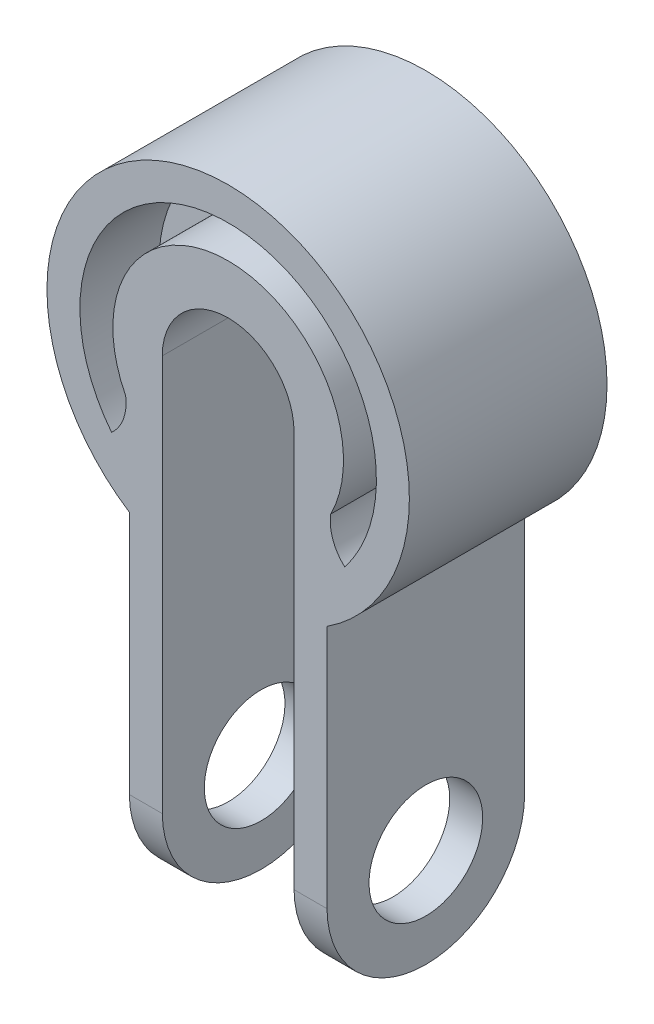
ISO-10303-21;
HEADER;
FILE_DESCRIPTION(('STEP AP214'),'2;1');
FILE_NAME('part.step','',(''),(''),'','','');
FILE_SCHEMA(('AUTOMOTIVE_DESIGN { 1 0 10303 214 1 1 1 1 }'));
ENDSEC;
DATA;
#1=APPLICATION_CONTEXT('core data for automotive mechanical design processes');
#2=APPLICATION_PROTOCOL_DEFINITION('international standard','automotive_design',2000,#1);
#3=PRODUCT_CONTEXT('',#1,'mechanical');
#4=PRODUCT('Part','Part','',(#3));
#5=PRODUCT_RELATED_PRODUCT_CATEGORY('part','',(#4));
#6=PRODUCT_DEFINITION_FORMATION('','',#4);
#7=PRODUCT_DEFINITION_CONTEXT('part definition',#1,'design');
#8=PRODUCT_DEFINITION('design','',#6,#7);
#9=PRODUCT_DEFINITION_SHAPE('','',#8);
#10=(LENGTH_UNIT() NAMED_UNIT(*) SI_UNIT(.MILLI.,.METRE.));
#11=(NAMED_UNIT(*) PLANE_ANGLE_UNIT() SI_UNIT($,.RADIAN.));
#12=(NAMED_UNIT(*) SI_UNIT($,.STERADIAN.) SOLID_ANGLE_UNIT());
#13=UNCERTAINTY_MEASURE_WITH_UNIT(LENGTH_MEASURE(1.E-05),#10,'distance_accuracy_value','');
#14=(GEOMETRIC_REPRESENTATION_CONTEXT(3) GLOBAL_UNCERTAINTY_ASSIGNED_CONTEXT((#13)) GLOBAL_UNIT_ASSIGNED_CONTEXT((#10,
#11,#12)) REPRESENTATION_CONTEXT('',''));
#15=CARTESIAN_POINT('',(0.,0.,0.));
#16=DIRECTION('',(0.,0.,1.));
#17=DIRECTION('',(1.,0.,0.));
#18=AXIS2_PLACEMENT_3D('',#15,#16,#17);
#19=CARTESIAN_POINT('',(15.,0.,15.));
#20=DIRECTION('',(1.,0.,0.));
#21=DIRECTION('',(0.,1.,0.));
#22=AXIS2_PLACEMENT_3D('',#19,#20,#21);
#23=PLANE('',#22);
#24=CARTESIAN_POINT('',(15.,-59.9991735844442,0.));
#25=DIRECTION('',(1.,0.,0.));
#26=DIRECTION('',(0.,1.,0.));
#27=AXIS2_PLACEMENT_3D('',#24,#25,#26);
#28=CIRCLE('',#27,8.62165443040973);
#29=CARTESIAN_POINT('',(15.,-51.3775191540345,0.));
#30=VERTEX_POINT('',#29);
#31=EDGE_CURVE('E249',#30,#30,#28,.T.);
#32=ORIENTED_EDGE('',*,*,#31,.F.);
#33=EDGE_LOOP('',(#32));
#34=FACE_BOUND('',#33,.T.);
#35=CARTESIAN_POINT('',(15.,-59.9991735844442,0.));
#36=DIRECTION('',(1.,0.,0.));
#37=DIRECTION('',(0.,1.,0.));
#38=AXIS2_PLACEMENT_3D('',#35,#36,#37);
#39=CIRCLE('',#38,15.0008264155558);
#40=CARTESIAN_POINT('',(15.,-60.1566319904984,-15.));
#41=VERTEX_POINT('',#40);
#42=CARTESIAN_POINT('',(15.,-60.1566319904984,15.));
#43=VERTEX_POINT('',#42);
#44=EDGE_CURVE('E184',#41,#43,#39,.F.);
#45=ORIENTED_EDGE('',*,*,#44,.F.);
#46=DIRECTION('',(0.,-1.,0.));
#47=VECTOR('',#46,1.);
#48=CARTESIAN_POINT('',(15.,0.,-15.));
#49=LINE('',#48,#47);
#50=CARTESIAN_POINT('',(15.,-23.0488611432322,-15.));
#51=VERTEX_POINT('',#50);
#52=EDGE_CURVE('E190',#51,#41,#49,.T.);
#53=ORIENTED_EDGE('',*,*,#52,.F.);
#54=DIRECTION('',(0.,0.,-1.));
#55=VECTOR('',#54,1.);
#56=CARTESIAN_POINT('',(15.,-23.0488611432322,15.));
#57=LINE('',#56,#55);
#58=CARTESIAN_POINT('',(15.,-23.0488611432322,15.));
#59=VERTEX_POINT('',#58);
#60=EDGE_CURVE('E12',#59,#51,#57,.T.);
#61=ORIENTED_EDGE('',*,*,#60,.F.);
#62=DIRECTION('',(0.,-1.,0.));
#63=VECTOR('',#62,1.);
#64=CARTESIAN_POINT('',(15.,0.,15.));
#65=LINE('',#64,#63);
#66=EDGE_CURVE('E189',#59,#43,#65,.T.);
#67=ORIENTED_EDGE('',*,*,#66,.T.);
#68=EDGE_LOOP('',(#45,#53,#61,#67));
#69=FACE_BOUND('',#68,.T.);
#70=ADVANCED_FACE('F72',(#34,#69),#23,.T.);
#71=CARTESIAN_POINT('',(-15.,0.,15.));
#72=DIRECTION('',(1.,0.,0.));
#73=DIRECTION('',(0.,1.,0.));
#74=AXIS2_PLACEMENT_3D('',#71,#72,#73);
#75=PLANE('',#74);
#76=CARTESIAN_POINT('',(-15.,-59.9991735844442,0.));
#77=DIRECTION('',(1.,0.,0.));
#78=DIRECTION('',(0.,1.,0.));
#79=AXIS2_PLACEMENT_3D('',#76,#77,#78);
#80=CIRCLE('',#79,8.62165443040973);
#81=CARTESIAN_POINT('',(-15.,-51.3775191540345,0.));
#82=VERTEX_POINT('',#81);
#83=EDGE_CURVE('E261',#82,#82,#80,.T.);
#84=ORIENTED_EDGE('',*,*,#83,.T.);
#85=EDGE_LOOP('',(#84));
#86=FACE_BOUND('',#85,.T.);
#87=DIRECTION('',(0.,-1.,0.));
#88=VECTOR('',#87,1.);
#89=CARTESIAN_POINT('',(-15.,0.,-15.));
#90=LINE('',#89,#88);
#91=CARTESIAN_POINT('',(-15.,-23.0488611432322,-15.));
#92=VERTEX_POINT('',#91);
#93=CARTESIAN_POINT('',(-15.,-60.1566319904984,-15.));
#94=VERTEX_POINT('',#93);
#95=EDGE_CURVE('E211',#92,#94,#90,.T.);
#96=ORIENTED_EDGE('',*,*,#95,.T.);
#97=CARTESIAN_POINT('',(-15.,-59.9991735844442,0.));
#98=DIRECTION('',(1.,0.,0.));
#99=DIRECTION('',(0.,1.,0.));
#100=AXIS2_PLACEMENT_3D('',#97,#98,#99);
#101=CIRCLE('',#100,15.0008264155558);
#102=CARTESIAN_POINT('',(-15.,-60.1566319904984,15.));
#103=VERTEX_POINT('',#102);
#104=EDGE_CURVE('E258',#94,#103,#101,.F.);
#105=ORIENTED_EDGE('',*,*,#104,.T.);
#106=DIRECTION('',(0.,-1.,0.));
#107=VECTOR('',#106,1.);
#108=CARTESIAN_POINT('',(-15.,0.,15.));
#109=LINE('',#108,#107);
#110=CARTESIAN_POINT('',(-15.,-23.0488611432322,15.));
#111=VERTEX_POINT('',#110);
#112=EDGE_CURVE('E238',#111,#103,#109,.T.);
#113=ORIENTED_EDGE('',*,*,#112,.F.);
#114=DIRECTION('',(0.,0.,-1.));
#115=VECTOR('',#114,1.);
#116=CARTESIAN_POINT('',(-15.,-23.0488611432322,15.));
#117=LINE('',#116,#115);
#118=EDGE_CURVE('E79',#111,#92,#117,.T.);
#119=ORIENTED_EDGE('',*,*,#118,.T.);
#120=EDGE_LOOP('',(#96,#105,#113,#119));
#121=FACE_BOUND('',#120,.T.);
#122=ADVANCED_FACE('F240',(#86,#121),#75,.F.);
#123=CARTESIAN_POINT('',(-10.,0.,15.));
#124=DIRECTION('',(1.,0.,0.));
#125=DIRECTION('',(0.,0.,-1.));
#126=AXIS2_PLACEMENT_3D('',#123,#124,#125);
#127=PLANE('',#126);
#128=CARTESIAN_POINT('',(-10.,-59.9991735844442,0.));
#129=DIRECTION('',(1.,0.,0.));
#130=DIRECTION('',(0.,0.,-1.));
#131=AXIS2_PLACEMENT_3D('',#128,#129,#130);
#132=CIRCLE('',#131,8.62165443040973);
#133=CARTESIAN_POINT('',(-10.,-59.9991735844442,-8.62165443040973));
#134=VERTEX_POINT('',#133);
#135=EDGE_CURVE('E256',#134,#134,#132,.T.);
#136=ORIENTED_EDGE('',*,*,#135,.F.);
#137=EDGE_LOOP('',(#136));
#138=FACE_BOUND('',#137,.T.);
#139=CARTESIAN_POINT('',(-10.,-59.9991735844442,0.));
#140=DIRECTION('',(1.,0.,0.));
#141=DIRECTION('',(0.,0.,-1.));
#142=AXIS2_PLACEMENT_3D('',#139,#140,#141);
#143=CIRCLE('',#142,15.0008264155558);
#144=CARTESIAN_POINT('',(-10.,-60.1566319904984,-15.));
#145=VERTEX_POINT('',#144);
#146=CARTESIAN_POINT('',(-10.,-60.1566319904984,15.));
#147=VERTEX_POINT('',#146);
#148=EDGE_CURVE('E255',#145,#147,#143,.F.);
#149=ORIENTED_EDGE('',*,*,#148,.F.);
#150=DIRECTION('',(0.,-1.,0.));
#151=VECTOR('',#150,1.);
#152=CARTESIAN_POINT('',(-10.,0.,-15.));
#153=LINE('',#152,#151);
#154=CARTESIAN_POINT('',(-10.,0.,-15.));
#155=VERTEX_POINT('',#154);
#156=EDGE_CURVE('E222',#155,#145,#153,.T.);
#157=ORIENTED_EDGE('',*,*,#156,.F.);
#158=DIRECTION('',(0.,0.,-1.));
#159=VECTOR('',#158,1.);
#160=CARTESIAN_POINT('',(-10.,0.,15.));
#161=LINE('',#160,#159);
#162=CARTESIAN_POINT('',(-10.,0.,15.));
#163=VERTEX_POINT('',#162);
#164=EDGE_CURVE('E233',#163,#155,#161,.T.);
#165=ORIENTED_EDGE('',*,*,#164,.F.);
#166=DIRECTION('',(0.,-1.,0.));
#167=VECTOR('',#166,1.);
#168=CARTESIAN_POINT('',(-10.,0.,15.));
#169=LINE('',#168,#167);
#170=EDGE_CURVE('E321',#163,#147,#169,.T.);
#171=ORIENTED_EDGE('',*,*,#170,.T.);
#172=EDGE_LOOP('',(#149,#157,#165,#171));
#173=FACE_BOUND('',#172,.T.);
#174=ADVANCED_FACE('F336',(#138,#173),#127,.T.);
#175=CARTESIAN_POINT('',(10.,0.,15.));
#176=DIRECTION('',(1.,0.,0.));
#177=DIRECTION('',(0.,0.,-1.));
#178=AXIS2_PLACEMENT_3D('',#175,#176,#177);
#179=PLANE('',#178);
#180=CARTESIAN_POINT('',(9.99999999999999,-59.9991735844442,0.));
#181=DIRECTION('',(1.,0.,0.));
#182=DIRECTION('',(0.,0.,-1.));
#183=AXIS2_PLACEMENT_3D('',#180,#181,#182);
#184=CIRCLE('',#183,8.62165443040973);
#185=CARTESIAN_POINT('',(9.99999999999999,-59.9991735844442,-8.62165443040973));
#186=VERTEX_POINT('',#185);
#187=EDGE_CURVE('E74',#186,#186,#184,.T.);
#188=ORIENTED_EDGE('',*,*,#187,.T.);
#189=EDGE_LOOP('',(#188));
#190=FACE_BOUND('',#189,.T.);
#191=DIRECTION('',(0.,-1.,0.));
#192=VECTOR('',#191,1.);
#193=CARTESIAN_POINT('',(10.,0.,-15.));
#194=LINE('',#193,#192);
#195=CARTESIAN_POINT('',(10.,0.,-15.));
#196=VERTEX_POINT('',#195);
#197=CARTESIAN_POINT('',(9.99999999999999,-60.1566319904984,-15.));
#198=VERTEX_POINT('',#197);
#199=EDGE_CURVE('E230',#196,#198,#194,.T.);
#200=ORIENTED_EDGE('',*,*,#199,.T.);
#201=CARTESIAN_POINT('',(9.99999999999999,-59.9991735844442,0.));
#202=DIRECTION('',(1.,0.,0.));
#203=DIRECTION('',(0.,0.,-1.));
#204=AXIS2_PLACEMENT_3D('',#201,#202,#203);
#205=CIRCLE('',#204,15.0008264155558);
#206=CARTESIAN_POINT('',(9.99999999999999,-60.1566319904984,15.));
#207=VERTEX_POINT('',#206);
#208=EDGE_CURVE('E200',#198,#207,#205,.F.);
#209=ORIENTED_EDGE('',*,*,#208,.T.);
#210=DIRECTION('',(0.,-1.,0.));
#211=VECTOR('',#210,1.);
#212=CARTESIAN_POINT('',(10.,0.,15.));
#213=LINE('',#212,#211);
#214=CARTESIAN_POINT('',(10.,0.,15.));
#215=VERTEX_POINT('',#214);
#216=EDGE_CURVE('E216',#215,#207,#213,.T.);
#217=ORIENTED_EDGE('',*,*,#216,.F.);
#218=DIRECTION('',(0.,0.,-1.));
#219=VECTOR('',#218,1.);
#220=CARTESIAN_POINT('',(10.,0.,15.));
#221=LINE('',#220,#219);
#222=EDGE_CURVE('E229',#215,#196,#221,.T.);
#223=ORIENTED_EDGE('',*,*,#222,.T.);
#224=EDGE_LOOP('',(#200,#209,#217,#223));
#225=FACE_BOUND('',#224,.T.);
#226=ADVANCED_FACE('F331',(#190,#225),#179,.F.);
#227=CARTESIAN_POINT('',(0.,0.,-15.));
#228=DIRECTION('',(0.,0.,1.));
#229=DIRECTION('',(1.,0.,0.));
#230=AXIS2_PLACEMENT_3D('',#227,#228,#229);
#231=PLANE('',#230);
#232=ORIENTED_EDGE('',*,*,#52,.T.);
#233=DIRECTION('',(1.,0.,0.));
#234=VECTOR('',#233,1.);
#235=CARTESIAN_POINT('',(-27.5,-60.1566319904984,-15.));
#236=LINE('',#235,#234);
#237=EDGE_CURVE('E198',#198,#41,#236,.T.);
#238=ORIENTED_EDGE('',*,*,#237,.F.);
#239=ORIENTED_EDGE('',*,*,#199,.F.);
#240=CARTESIAN_POINT('',(0.,0.,-15.));
#241=DIRECTION('',(0.,0.,1.));
#242=DIRECTION('',(1.,0.,0.));
#243=AXIS2_PLACEMENT_3D('',#240,#241,#242);
#244=CIRCLE('',#243,10.);
#245=EDGE_CURVE('E221',#196,#155,#244,.T.);
#246=ORIENTED_EDGE('',*,*,#245,.T.);
#247=ORIENTED_EDGE('',*,*,#156,.T.);
#248=EDGE_CURVE('E191',#94,#145,#236,.T.);
#249=ORIENTED_EDGE('',*,*,#248,.F.);
#250=ORIENTED_EDGE('',*,*,#95,.F.);
#251=CARTESIAN_POINT('',(0.,0.,-15.));
#252=DIRECTION('',(0.,0.,1.));
#253=DIRECTION('',(1.,0.,0.));
#254=AXIS2_PLACEMENT_3D('',#251,#252,#253);
#255=CIRCLE('',#254,27.5);
#256=EDGE_CURVE('E208',#51,#92,#255,.T.);
#257=ORIENTED_EDGE('',*,*,#256,.F.);
#258=EDGE_LOOP('',(#232,#238,#239,#246,#247,#249,#250,#257));
#259=FACE_BOUND('',#258,.T.);
#260=CARTESIAN_POINT('',(-22.1733590483481,-8.94396020159915,-15.));
#261=DIRECTION('',(0.,0.,1.));
#262=DIRECTION('',(1.,0.,0.));
#263=AXIS2_PLACEMENT_3D('',#260,#261,#262);
#264=CIRCLE('',#263,6.68110355015165);
#265=CARTESIAN_POINT('',(-17.6929073651534,-13.9000370131918,-15.));
#266=VERTEX_POINT('',#265);
#267=CARTESIAN_POINT('',(-15.5573371379465,-8.01369210640574,-15.));
#268=VERTEX_POINT('',#267);
#269=EDGE_CURVE('E277',#266,#268,#264,.T.);
#270=ORIENTED_EDGE('',*,*,#269,.T.);
#271=CARTESIAN_POINT('',(0.,0.,-15.));
#272=DIRECTION('',(0.,0.,1.));
#273=DIRECTION('',(1.,0.,0.));
#274=AXIS2_PLACEMENT_3D('',#271,#272,#273);
#275=CIRCLE('',#274,17.5);
#276=CARTESIAN_POINT('',(15.5573371379465,-8.01369210640575,-15.));
#277=VERTEX_POINT('',#276);
#278=EDGE_CURVE('E88',#277,#268,#275,.T.);
#279=ORIENTED_EDGE('',*,*,#278,.F.);
#280=CARTESIAN_POINT('',(22.1733590483481,-8.94396020159914,-15.));
#281=DIRECTION('',(0.,0.,1.));
#282=DIRECTION('',(1.,0.,0.));
#283=AXIS2_PLACEMENT_3D('',#280,#281,#282);
#284=CIRCLE('',#283,6.68110355015165);
#285=CARTESIAN_POINT('',(17.6929073651534,-13.9000370131918,-15.));
#286=VERTEX_POINT('',#285);
#287=EDGE_CURVE('E268',#277,#286,#284,.T.);
#288=ORIENTED_EDGE('',*,*,#287,.T.);
#289=CARTESIAN_POINT('',(0.,0.,-15.));
#290=DIRECTION('',(0.,0.,1.));
#291=DIRECTION('',(1.,0.,0.));
#292=AXIS2_PLACEMENT_3D('',#289,#290,#291);
#293=CIRCLE('',#292,22.5);
#294=EDGE_CURVE('E276',#286,#266,#293,.T.);
#295=ORIENTED_EDGE('',*,*,#294,.T.);
#296=EDGE_LOOP('',(#270,#279,#288,#295));
#297=FACE_BOUND('',#296,.T.);
#298=ADVANCED_FACE('F202',(#259,#297),#231,.F.);
#299=CARTESIAN_POINT('',(0.,0.,15.));
#300=DIRECTION('',(0.,0.,1.));
#301=DIRECTION('',(1.,0.,0.));
#302=AXIS2_PLACEMENT_3D('',#299,#300,#301);
#303=PLANE('',#302);
#304=DIRECTION('',(1.,0.,0.));
#305=VECTOR('',#304,1.);
#306=CARTESIAN_POINT('',(-27.5,-60.1566319904984,15.));
#307=LINE('',#306,#305);
#308=EDGE_CURVE('E195',#207,#43,#307,.T.);
#309=ORIENTED_EDGE('',*,*,#308,.T.);
#310=ORIENTED_EDGE('',*,*,#66,.F.);
#311=CARTESIAN_POINT('',(0.,0.,15.));
#312=DIRECTION('',(0.,0.,1.));
#313=DIRECTION('',(1.,0.,0.));
#314=AXIS2_PLACEMENT_3D('',#311,#312,#313);
#315=CIRCLE('',#314,27.5);
#316=EDGE_CURVE('E318',#59,#111,#315,.T.);
#317=ORIENTED_EDGE('',*,*,#316,.T.);
#318=ORIENTED_EDGE('',*,*,#112,.T.);
#319=EDGE_CURVE('E247',#103,#147,#307,.T.);
#320=ORIENTED_EDGE('',*,*,#319,.T.);
#321=ORIENTED_EDGE('',*,*,#170,.F.);
#322=CARTESIAN_POINT('',(0.,0.,15.));
#323=DIRECTION('',(0.,0.,1.));
#324=DIRECTION('',(1.,0.,0.));
#325=AXIS2_PLACEMENT_3D('',#322,#323,#324);
#326=CIRCLE('',#325,10.);
#327=EDGE_CURVE('E323',#215,#163,#326,.T.);
#328=ORIENTED_EDGE('',*,*,#327,.F.);
#329=ORIENTED_EDGE('',*,*,#216,.T.);
#330=EDGE_LOOP('',(#309,#310,#317,#318,#320,#321,#328,#329));
#331=FACE_BOUND('',#330,.T.);
#332=CARTESIAN_POINT('',(22.1733590483481,-8.94396020159914,15.));
#333=DIRECTION('',(0.,0.,1.));
#334=DIRECTION('',(1.,0.,0.));
#335=AXIS2_PLACEMENT_3D('',#332,#333,#334);
#336=CIRCLE('',#335,6.68110355015165);
#337=CARTESIAN_POINT('',(15.5573371379465,-8.01369210640575,15.));
#338=VERTEX_POINT('',#337);
#339=CARTESIAN_POINT('',(17.6929073651534,-13.9000370131918,15.));
#340=VERTEX_POINT('',#339);
#341=EDGE_CURVE('E294',#338,#340,#336,.T.);
#342=ORIENTED_EDGE('',*,*,#341,.F.);
#343=CARTESIAN_POINT('',(0.,0.,15.));
#344=DIRECTION('',(0.,0.,1.));
#345=DIRECTION('',(1.,0.,0.));
#346=AXIS2_PLACEMENT_3D('',#343,#344,#345);
#347=CIRCLE('',#346,17.5);
#348=CARTESIAN_POINT('',(-15.5573371379465,-8.01369210640574,15.));
#349=VERTEX_POINT('',#348);
#350=EDGE_CURVE('E94',#338,#349,#347,.T.);
#351=ORIENTED_EDGE('',*,*,#350,.T.);
#352=CARTESIAN_POINT('',(-22.1733590483481,-8.94396020159915,15.));
#353=DIRECTION('',(0.,0.,1.));
#354=DIRECTION('',(1.,0.,0.));
#355=AXIS2_PLACEMENT_3D('',#352,#353,#354);
#356=CIRCLE('',#355,6.68110355015165);
#357=CARTESIAN_POINT('',(-17.6929073651534,-13.9000370131918,15.));
#358=VERTEX_POINT('',#357);
#359=EDGE_CURVE('E304',#358,#349,#356,.T.);
#360=ORIENTED_EDGE('',*,*,#359,.F.);
#361=CARTESIAN_POINT('',(0.,0.,15.));
#362=DIRECTION('',(0.,0.,1.));
#363=DIRECTION('',(1.,0.,0.));
#364=AXIS2_PLACEMENT_3D('',#361,#362,#363);
#365=CIRCLE('',#364,22.5);
#366=EDGE_CURVE('E306',#340,#358,#365,.T.);
#367=ORIENTED_EDGE('',*,*,#366,.F.);
#368=EDGE_LOOP('',(#342,#351,#360,#367));
#369=FACE_BOUND('',#368,.T.);
#370=ADVANCED_FACE('F329',(#331,#369),#303,.T.);
#371=CARTESIAN_POINT('',(0.,0.,15.));
#372=DIRECTION('',(0.,0.,-1.));
#373=DIRECTION('',(-1.,0.,0.));
#374=AXIS2_PLACEMENT_3D('',#371,#372,#373);
#375=CYLINDRICAL_SURFACE('',#374,27.5);
#376=ORIENTED_EDGE('',*,*,#256,.T.);
#377=ORIENTED_EDGE('',*,*,#118,.F.);
#378=ORIENTED_EDGE('',*,*,#316,.F.);
#379=ORIENTED_EDGE('',*,*,#60,.T.);
#380=EDGE_LOOP('',(#376,#377,#378,#379));
#381=FACE_BOUND('',#380,.T.);
#382=ADVANCED_FACE('F343',(#381),#375,.T.);
#383=CARTESIAN_POINT('',(0.,0.,15.));
#384=DIRECTION('',(0.,0.,-1.));
#385=DIRECTION('',(-1.,0.,0.));
#386=AXIS2_PLACEMENT_3D('',#383,#384,#385);
#387=CYLINDRICAL_SURFACE('',#386,10.);
#388=ORIENTED_EDGE('',*,*,#245,.F.);
#389=ORIENTED_EDGE('',*,*,#222,.F.);
#390=ORIENTED_EDGE('',*,*,#327,.T.);
#391=ORIENTED_EDGE('',*,*,#164,.T.);
#392=EDGE_LOOP('',(#388,#389,#390,#391));
#393=FACE_BOUND('',#392,.T.);
#394=ADVANCED_FACE('F338',(#393),#387,.F.);
#395=CARTESIAN_POINT('',(0.,0.,3.));
#396=DIRECTION('',(0.,0.,1.));
#397=DIRECTION('',(1.,0.,0.));
#398=AXIS2_PLACEMENT_3D('',#395,#396,#397);
#399=CYLINDRICAL_SURFACE('',#398,17.5);
#400=ORIENTED_EDGE('',*,*,#350,.F.);
#401=DIRECTION('',(0.,0.,1.));
#402=VECTOR('',#401,1.);
#403=CARTESIAN_POINT('',(15.5573371379465,-8.01369210640575,3.));
#404=LINE('',#403,#402);
#405=CARTESIAN_POINT('',(15.5573371379465,-8.01369210640575,3.));
#406=VERTEX_POINT('',#405);
#407=EDGE_CURVE('E301',#406,#338,#404,.T.);
#408=ORIENTED_EDGE('',*,*,#407,.F.);
#409=CARTESIAN_POINT('',(0.,0.,3.));
#410=DIRECTION('',(0.,0.,1.));
#411=DIRECTION('',(1.,0.,0.));
#412=AXIS2_PLACEMENT_3D('',#409,#410,#411);
#413=CIRCLE('',#412,17.5);
#414=CARTESIAN_POINT('',(-15.5573371379465,-8.01369210640574,3.));
#415=VERTEX_POINT('',#414);
#416=EDGE_CURVE('E292',#406,#415,#413,.T.);
#417=ORIENTED_EDGE('',*,*,#416,.T.);
#418=DIRECTION('',(0.,0.,1.));
#419=VECTOR('',#418,1.);
#420=CARTESIAN_POINT('',(-15.5573371379465,-8.01369210640574,3.));
#421=LINE('',#420,#419);
#422=EDGE_CURVE('E207',#415,#349,#421,.T.);
#423=ORIENTED_EDGE('',*,*,#422,.T.);
#424=EDGE_LOOP('',(#400,#408,#417,#423));
#425=FACE_BOUND('',#424,.T.);
#426=ADVANCED_FACE('F350',(#425),#399,.T.);
#427=CARTESIAN_POINT('',(-22.1733590483481,-8.94396020159915,3.));
#428=DIRECTION('',(0.,0.,1.));
#429=DIRECTION('',(1.,0.,0.));
#430=AXIS2_PLACEMENT_3D('',#427,#428,#429);
#431=CYLINDRICAL_SURFACE('',#430,6.68110355015165);
#432=ORIENTED_EDGE('',*,*,#359,.T.);
#433=ORIENTED_EDGE('',*,*,#422,.F.);
#434=CARTESIAN_POINT('',(-22.1733590483481,-8.94396020159915,3.));
#435=DIRECTION('',(0.,0.,1.));
#436=DIRECTION('',(1.,0.,0.));
#437=AXIS2_PLACEMENT_3D('',#434,#435,#436);
#438=CIRCLE('',#437,6.68110355015165);
#439=CARTESIAN_POINT('',(-17.6929073651534,-13.9000370131918,3.));
#440=VERTEX_POINT('',#439);
#441=EDGE_CURVE('E291',#440,#415,#438,.T.);
#442=ORIENTED_EDGE('',*,*,#441,.F.);
#443=DIRECTION('',(0.,0.,1.));
#444=VECTOR('',#443,1.);
#445=CARTESIAN_POINT('',(-17.6929073651534,-13.9000370131918,3.));
#446=LINE('',#445,#444);
#447=EDGE_CURVE('E213',#440,#358,#446,.T.);
#448=ORIENTED_EDGE('',*,*,#447,.T.);
#449=EDGE_LOOP('',(#432,#433,#442,#448));
#450=FACE_BOUND('',#449,.T.);
#451=ADVANCED_FACE('F377',(#450),#431,.F.);
#452=CARTESIAN_POINT('',(0.,0.,3.));
#453=DIRECTION('',(0.,0.,1.));
#454=DIRECTION('',(1.,0.,0.));
#455=AXIS2_PLACEMENT_3D('',#452,#453,#454);
#456=CYLINDRICAL_SURFACE('',#455,22.5);
#457=ORIENTED_EDGE('',*,*,#366,.T.);
#458=ORIENTED_EDGE('',*,*,#447,.F.);
#459=CARTESIAN_POINT('',(0.,0.,3.));
#460=DIRECTION('',(0.,0.,1.));
#461=DIRECTION('',(1.,0.,0.));
#462=AXIS2_PLACEMENT_3D('',#459,#460,#461);
#463=CIRCLE('',#462,22.5);
#464=CARTESIAN_POINT('',(17.6929073651534,-13.9000370131918,3.));
#465=VERTEX_POINT('',#464);
#466=EDGE_CURVE('E300',#465,#440,#463,.T.);
#467=ORIENTED_EDGE('',*,*,#466,.F.);
#468=DIRECTION('',(0.,0.,1.));
#469=VECTOR('',#468,1.);
#470=CARTESIAN_POINT('',(17.6929073651534,-13.9000370131918,3.));
#471=LINE('',#470,#469);
#472=EDGE_CURVE('E314',#465,#340,#471,.T.);
#473=ORIENTED_EDGE('',*,*,#472,.T.);
#474=EDGE_LOOP('',(#457,#458,#467,#473));
#475=FACE_BOUND('',#474,.T.);
#476=ADVANCED_FACE('F385',(#475),#456,.F.);
#477=CARTESIAN_POINT('',(22.1733590483481,-8.94396020159914,3.));
#478=DIRECTION('',(0.,0.,1.));
#479=DIRECTION('',(1.,0.,0.));
#480=AXIS2_PLACEMENT_3D('',#477,#478,#479);
#481=CYLINDRICAL_SURFACE('',#480,6.68110355015165);
#482=ORIENTED_EDGE('',*,*,#341,.T.);
#483=ORIENTED_EDGE('',*,*,#472,.F.);
#484=CARTESIAN_POINT('',(22.1733590483481,-8.94396020159914,3.));
#485=DIRECTION('',(0.,0.,1.));
#486=DIRECTION('',(1.,0.,0.));
#487=AXIS2_PLACEMENT_3D('',#484,#485,#486);
#488=CIRCLE('',#487,6.68110355015165);
#489=EDGE_CURVE('E297',#406,#465,#488,.T.);
#490=ORIENTED_EDGE('',*,*,#489,.F.);
#491=ORIENTED_EDGE('',*,*,#407,.T.);
#492=EDGE_LOOP('',(#482,#483,#490,#491));
#493=FACE_BOUND('',#492,.T.);
#494=ADVANCED_FACE('F387',(#493),#481,.F.);
#495=CARTESIAN_POINT('',(-11.0866795241741,-4.47198010079957,3.));
#496=DIRECTION('',(0.,0.,1.));
#497=DIRECTION('',(1.,0.,0.));
#498=AXIS2_PLACEMENT_3D('',#495,#496,#497);
#499=PLANE('',#498);
#500=ORIENTED_EDGE('',*,*,#416,.F.);
#501=ORIENTED_EDGE('',*,*,#489,.T.);
#502=ORIENTED_EDGE('',*,*,#466,.T.);
#503=ORIENTED_EDGE('',*,*,#441,.T.);
#504=EDGE_LOOP('',(#500,#501,#502,#503));
#505=FACE_BOUND('',#504,.T.);
#506=ADVANCED_FACE('F388',(#505),#499,.T.);
#507=CARTESIAN_POINT('',(0.,0.,-3.));
#508=DIRECTION('',(0.,0.,-1.));
#509=DIRECTION('',(-1.,0.,0.));
#510=AXIS2_PLACEMENT_3D('',#507,#508,#509);
#511=CYLINDRICAL_SURFACE('',#510,17.5);
#512=ORIENTED_EDGE('',*,*,#278,.T.);
#513=DIRECTION('',(0.,0.,-1.));
#514=VECTOR('',#513,1.);
#515=CARTESIAN_POINT('',(-15.5573371379465,-8.01369210640574,-3.));
#516=LINE('',#515,#514);
#517=CARTESIAN_POINT('',(-15.5573371379465,-8.01369210640574,-3.));
#518=VERTEX_POINT('',#517);
#519=EDGE_CURVE('E273',#518,#268,#516,.T.);
#520=ORIENTED_EDGE('',*,*,#519,.F.);
#521=CARTESIAN_POINT('',(0.,0.,-3.));
#522=DIRECTION('',(0.,0.,1.));
#523=DIRECTION('',(1.,0.,0.));
#524=AXIS2_PLACEMENT_3D('',#521,#522,#523);
#525=CIRCLE('',#524,17.5);
#526=CARTESIAN_POINT('',(15.5573371379465,-8.01369210640575,-3.));
#527=VERTEX_POINT('',#526);
#528=EDGE_CURVE('E262',#527,#518,#525,.T.);
#529=ORIENTED_EDGE('',*,*,#528,.F.);
#530=DIRECTION('',(0.,0.,-1.));
#531=VECTOR('',#530,1.);
#532=CARTESIAN_POINT('',(15.5573371379465,-8.01369210640575,-3.));
#533=LINE('',#532,#531);
#534=EDGE_CURVE('E284',#527,#277,#533,.T.);
#535=ORIENTED_EDGE('',*,*,#534,.T.);
#536=EDGE_LOOP('',(#512,#520,#529,#535));
#537=FACE_BOUND('',#536,.T.);
#538=ADVANCED_FACE('F394',(#537),#511,.T.);
#539=CARTESIAN_POINT('',(22.1733590483481,-8.94396020159914,-3.));
#540=DIRECTION('',(0.,0.,-1.));
#541=DIRECTION('',(-1.,0.,0.));
#542=AXIS2_PLACEMENT_3D('',#539,#540,#541);
#543=CYLINDRICAL_SURFACE('',#542,6.68110355015165);
#544=ORIENTED_EDGE('',*,*,#287,.F.);
#545=ORIENTED_EDGE('',*,*,#534,.F.);
#546=CARTESIAN_POINT('',(22.1733590483481,-8.94396020159914,-3.));
#547=DIRECTION('',(0.,0.,1.));
#548=DIRECTION('',(1.,0.,0.));
#549=AXIS2_PLACEMENT_3D('',#546,#547,#548);
#550=CIRCLE('',#549,6.68110355015165);
#551=CARTESIAN_POINT('',(17.6929073651534,-13.9000370131918,-3.));
#552=VERTEX_POINT('',#551);
#553=EDGE_CURVE('E275',#527,#552,#550,.T.);
#554=ORIENTED_EDGE('',*,*,#553,.T.);
#555=DIRECTION('',(0.,0.,-1.));
#556=VECTOR('',#555,1.);
#557=CARTESIAN_POINT('',(17.6929073651534,-13.9000370131918,-3.));
#558=LINE('',#557,#556);
#559=EDGE_CURVE('E288',#552,#286,#558,.T.);
#560=ORIENTED_EDGE('',*,*,#559,.T.);
#561=EDGE_LOOP('',(#544,#545,#554,#560));
#562=FACE_BOUND('',#561,.T.);
#563=ADVANCED_FACE('F396',(#562),#543,.F.);
#564=CARTESIAN_POINT('',(0.,0.,-3.));
#565=DIRECTION('',(0.,0.,-1.));
#566=DIRECTION('',(-1.,0.,0.));
#567=AXIS2_PLACEMENT_3D('',#564,#565,#566);
#568=CYLINDRICAL_SURFACE('',#567,22.5);
#569=ORIENTED_EDGE('',*,*,#294,.F.);
#570=ORIENTED_EDGE('',*,*,#559,.F.);
#571=CARTESIAN_POINT('',(0.,0.,-3.));
#572=DIRECTION('',(0.,0.,1.));
#573=DIRECTION('',(1.,0.,0.));
#574=AXIS2_PLACEMENT_3D('',#571,#572,#573);
#575=CIRCLE('',#574,22.5);
#576=CARTESIAN_POINT('',(-17.6929073651534,-13.9000370131918,-3.));
#577=VERTEX_POINT('',#576);
#578=EDGE_CURVE('E269',#552,#577,#575,.T.);
#579=ORIENTED_EDGE('',*,*,#578,.T.);
#580=DIRECTION('',(0.,0.,-1.));
#581=VECTOR('',#580,1.);
#582=CARTESIAN_POINT('',(-17.6929073651534,-13.9000370131918,-3.));
#583=LINE('',#582,#581);
#584=EDGE_CURVE('E286',#577,#266,#583,.T.);
#585=ORIENTED_EDGE('',*,*,#584,.T.);
#586=EDGE_LOOP('',(#569,#570,#579,#585));
#587=FACE_BOUND('',#586,.T.);
#588=ADVANCED_FACE('F401',(#587),#568,.F.);
#589=CARTESIAN_POINT('',(-22.1733590483481,-8.94396020159915,-3.));
#590=DIRECTION('',(0.,0.,-1.));
#591=DIRECTION('',(-1.,0.,0.));
#592=AXIS2_PLACEMENT_3D('',#589,#590,#591);
#593=CYLINDRICAL_SURFACE('',#592,6.68110355015165);
#594=ORIENTED_EDGE('',*,*,#269,.F.);
#595=ORIENTED_EDGE('',*,*,#584,.F.);
#596=CARTESIAN_POINT('',(-22.1733590483481,-8.94396020159915,-3.));
#597=DIRECTION('',(0.,0.,1.));
#598=DIRECTION('',(1.,0.,0.));
#599=AXIS2_PLACEMENT_3D('',#596,#597,#598);
#600=CIRCLE('',#599,6.68110355015165);
#601=EDGE_CURVE('E270',#577,#518,#600,.T.);
#602=ORIENTED_EDGE('',*,*,#601,.T.);
#603=ORIENTED_EDGE('',*,*,#519,.T.);
#604=EDGE_LOOP('',(#594,#595,#602,#603));
#605=FACE_BOUND('',#604,.T.);
#606=ADVANCED_FACE('F397',(#605),#593,.F.);
#607=CARTESIAN_POINT('',(-11.0866795241741,-4.47198010079957,-3.));
#608=DIRECTION('',(0.,0.,1.));
#609=DIRECTION('',(1.,0.,0.));
#610=AXIS2_PLACEMENT_3D('',#607,#608,#609);
#611=PLANE('',#610);
#612=ORIENTED_EDGE('',*,*,#528,.T.);
#613=ORIENTED_EDGE('',*,*,#601,.F.);
#614=ORIENTED_EDGE('',*,*,#578,.F.);
#615=ORIENTED_EDGE('',*,*,#553,.F.);
#616=EDGE_LOOP('',(#612,#613,#614,#615));
#617=FACE_BOUND('',#616,.T.);
#618=ADVANCED_FACE('F405',(#617),#611,.F.);
#619=CARTESIAN_POINT('',(-27.5,-59.9991735844442,0.));
#620=DIRECTION('',(1.,0.,0.));
#621=DIRECTION('',(0.,1.,0.));
#622=AXIS2_PLACEMENT_3D('',#619,#620,#621);
#623=CYLINDRICAL_SURFACE('',#622,15.0008264155558);
#624=ORIENTED_EDGE('',*,*,#208,.F.);
#625=ORIENTED_EDGE('',*,*,#237,.T.);
#626=ORIENTED_EDGE('',*,*,#44,.T.);
#627=ORIENTED_EDGE('',*,*,#308,.F.);
#628=EDGE_LOOP('',(#624,#625,#626,#627));
#629=FACE_BOUND('',#628,.T.);
#630=ADVANCED_FACE('F197',(#629),#623,.T.);
#631=CARTESIAN_POINT('',(-27.5,-59.9991735844442,0.));
#632=DIRECTION('',(1.,0.,0.));
#633=DIRECTION('',(0.,1.,0.));
#634=AXIS2_PLACEMENT_3D('',#631,#632,#633);
#635=CYLINDRICAL_SURFACE('',#634,8.62165443040973);
#636=ORIENTED_EDGE('',*,*,#31,.T.);
#637=EDGE_LOOP('',(#636));
#638=FACE_BOUND('',#637,.T.);
#639=ORIENTED_EDGE('',*,*,#187,.F.);
#640=EDGE_LOOP('',(#639));
#641=FACE_BOUND('',#640,.T.);
#642=ADVANCED_FACE('F357',(#638,#641),#635,.F.);
#643=ORIENTED_EDGE('',*,*,#135,.T.);
#644=EDGE_LOOP('',(#643));
#645=FACE_BOUND('',#644,.T.);
#646=ORIENTED_EDGE('',*,*,#83,.F.);
#647=EDGE_LOOP('',(#646));
#648=FACE_BOUND('',#647,.T.);
#649=ADVANCED_FACE('F362',(#645,#648),#635,.F.);
#650=ORIENTED_EDGE('',*,*,#104,.F.);
#651=ORIENTED_EDGE('',*,*,#248,.T.);
#652=ORIENTED_EDGE('',*,*,#148,.T.);
#653=ORIENTED_EDGE('',*,*,#319,.F.);
#654=EDGE_LOOP('',(#650,#651,#652,#653));
#655=FACE_BOUND('',#654,.T.);
#656=ADVANCED_FACE('F337',(#655),#623,.T.);
#657=CLOSED_SHELL('',(#70,#122,#174,#226,#298,#370,#382,#394,#426,#451,#476,#494,#506,#538,#563,
#588,#606,#618,#630,#642,#649,#656));
#658=MANIFOLD_SOLID_BREP('B2',#657);
#659=ADVANCED_BREP_SHAPE_REPRESENTATION('',(#18,#658),#14);
#660=SHAPE_DEFINITION_REPRESENTATION(#9,#659);
ENDSEC;
END-ISO-10303-21;
